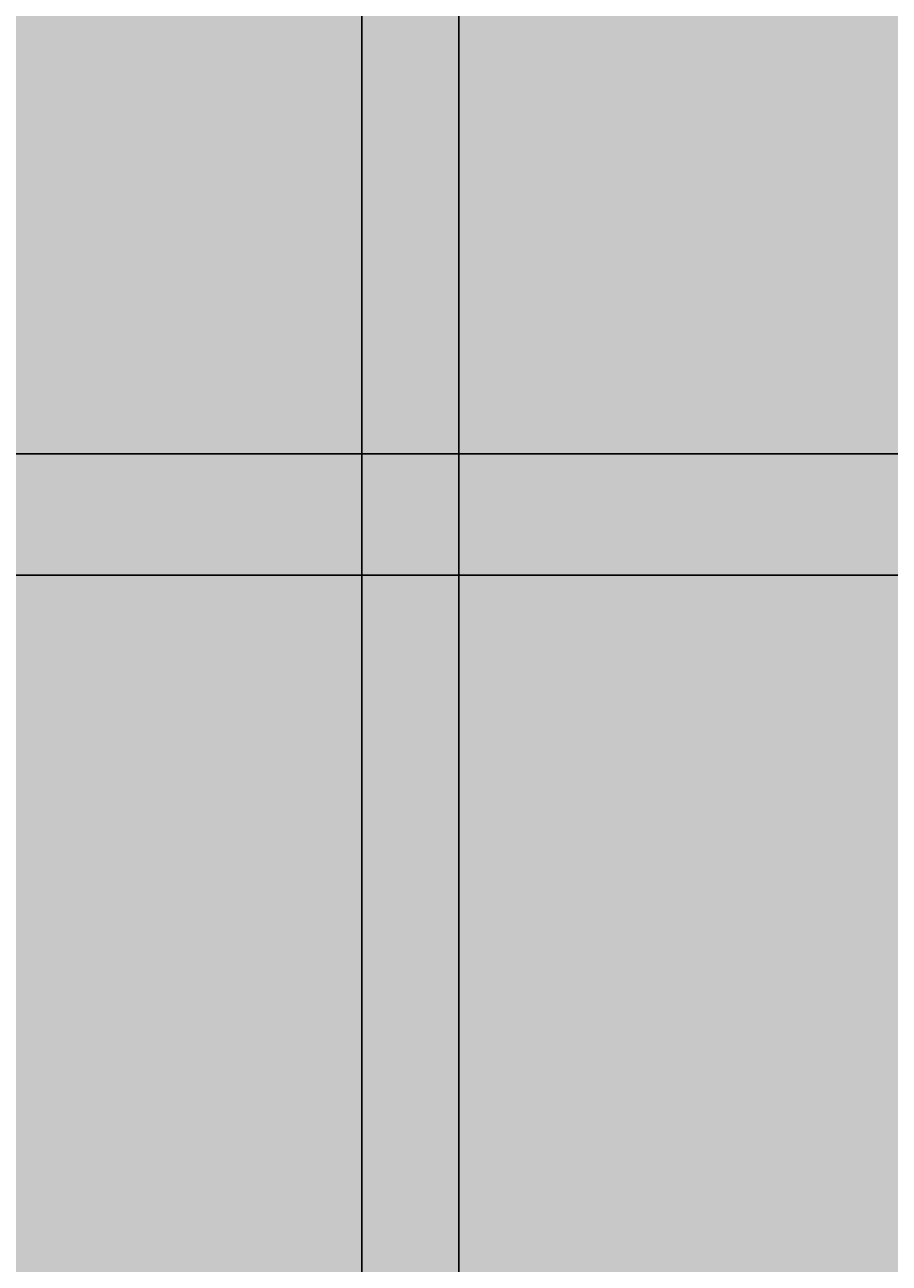
# Model space of a CAD drawing. Units: inches. Extents: x -12 to 334, y -10 to 186.
# Tile 65 of 77: x 239 to 257, y 111 to 137. Entities that reach past the tile are written whole.
import ezdxf

# ---------------------------------------------------------------- set-up
doc = ezdxf.new("R2010")
doc.units = ezdxf.units.IN
doc.header["$MEASUREMENT"] = 0
doc.layers.add('M-DIMS', color=2, linetype='Continuous', lineweight=18)
doc.layers.add('M-EQPM-PATT', color=8, linetype='Continuous', lineweight=18)
doc.styles.get("Standard").update_dxf_attribs({"font": 'arial.ttf'})
doc.dimstyles.get("Standard").update_dxf_attribs({"dimtxt": 0.18, "dimasz": 0.18, "dimexe": 0.18, "dimexo": 0.0625, "dimgap": 0.09, "dimtad": 0, "dimtih": 1, "dimtoh": 1, "dimdec": 4, "dimzin": 0, "dimdsep": 46, "dimtxsty": 'Standard', "dimcen": 0.09, "dimadec": 0, "dimazin": 0, "dimtfac": 1, "dimtdec": 4, "dimtofl": 0, "dimtmove": 0, "dimatfit": 3, "dimfxl": 1, "dimtolj": 1, "dimtzin": 0, "dimarcsym": 0})

# ---------------------------------------------------------------- blocks, each defined once
blk = doc.blocks.new('*D5')
at = {"layer": 'Defpoints', "color": 0, "transparency": 16777216}
for p in [(58.1, 127.708), (58.1, 125.208), (295.976, 125.208)]:
    blk.add_point(p, dxfattribs=at)
at = {"layer": 'M-DIMS', "color": 0, "lineweight": -2, "transparency": 16777216}
for p, q in [((58.163, 127.708), (296.156, 127.708)), ((295.976, 127.528), (295.976, 126.64)), ((295.976, 125.388), (295.976, 126.276)), ((58.163, 125.208), (296.156, 125.208))]:
    blk.add_line(p, q, dxfattribs=at)
at = {"layer": 'M-DIMS', "color": 0, "transparency": 16777216}
for points in [[(295.946, 127.528), (296.006, 127.528), (295.976, 127.708)], [(295.946, 125.388), (296.006, 125.388), (295.976, 125.208)]]:
    blk.add_solid(points, dxfattribs=at)
at = {"layer": 'M-DIMS', "color": 0, "transparency": 16777216, "insert": (295.976, 126.458), "char_height": 0.18, "attachment_point": 5}
blk.add_mtext('\\A1;2.5', dxfattribs=at)
blk = doc.blocks.new('*D36')
at = {"layer": 'Defpoints', "color": 0, "transparency": 16777216}
for p in [(247.935, 169.385), (245.935, 82.697), (247.935, 82.697)]:
    blk.add_point(p, dxfattribs=at)
at = {"layer": 'M-DIMS', "color": 0, "lineweight": -2, "transparency": 16777216}
for p, q in [((245.935, 82.759), (245.935, 169.565)), ((247.935, 82.759), (247.935, 169.565)), ((246.115, 169.385), (246.786, 169.385)), ((247.755, 169.385), (247.085, 169.385))]:
    blk.add_line(p, q, dxfattribs=at)
at = {"layer": 'M-DIMS', "color": 0, "transparency": 16777216}
for points in [[(246.115, 169.415), (246.115, 169.355), (245.935, 169.385)], [(247.755, 169.415), (247.755, 169.355), (247.935, 169.385)]]:
    blk.add_solid(points, dxfattribs=at)
at = {"layer": 'M-DIMS', "color": 0, "transparency": 16777216, "insert": (246.935, 169.385), "char_height": 0.18, "attachment_point": 5}
blk.add_mtext('\\A1;2', dxfattribs=at)
blk = doc.blocks.new('*D37')
at = {"layer": 'Defpoints', "color": 0, "transparency": 16777216}
for p in [(245.935, 169.385), (232.576, 46.854), (245.935, 46.854)]:
    blk.add_point(p, dxfattribs=at)
at = {"layer": 'M-DIMS', "color": 0, "lineweight": -2, "transparency": 16777216}
for p, q in [((232.576, 46.917), (232.576, 169.565)), ((245.935, 46.917), (245.935, 169.565)), ((232.756, 169.385), (238.871, 169.385)), ((245.755, 169.385), (239.641, 169.385))]:
    blk.add_line(p, q, dxfattribs=at)
at = {"layer": 'M-DIMS', "color": 0, "transparency": 16777216}
for points in [[(232.756, 169.415), (232.756, 169.355), (232.576, 169.385)], [(245.755, 169.415), (245.755, 169.355), (245.935, 169.385)]]:
    blk.add_solid(points, dxfattribs=at)
at = {"layer": 'M-DIMS', "color": 0, "transparency": 16777216, "insert": (239.256, 169.385), "char_height": 0.18, "attachment_point": 5}
blk.add_mtext('\\A1;13.36', dxfattribs=at)
blk = doc.blocks.new('*D40')
at = {"layer": 'Defpoints', "color": 0, "transparency": 16777216}
for p in [(278.229, 116.208), (187.394, 91.899)]:
    blk.add_point(p, dxfattribs=at)
at = {"layer": 'M-DIMS', "color": 0, "lineweight": -2, "transparency": 16777216}
for p, q in [((332.73, 130.793), (278.403, 116.254)), ((187.394, 91.809), (187.394, 91.989)), ((187.304, 91.899), (187.484, 91.899))]:
    blk.add_line(p, q, dxfattribs=at)
at = {"layer": 'M-DIMS', "color": 0, "transparency": 16777216}
blk.add_solid([(278.395, 116.283), (278.411, 116.225), (278.229, 116.208)], dxfattribs=at)
at = {"layer": 'M-DIMS', "color": 0, "transparency": 16777216, "insert": (333.21, 130.793), "char_height": 0.18, "attachment_point": 5}
blk.add_mtext('\\A1;R94.03', dxfattribs=at)

msp = doc.modelspace()

# ---------------------------------------------------------------- hatches: boundary and pattern name
at = {"layer": 'M-EQPM-PATT', "transparency": 33554556}
h = msp.add_hatch(color=256, dxfattribs=at)
h.set_gradient(color1=(248, 206, 179), color2=(248, 206, 179), tint=1)
h.paths.add_polyline_path([(179.7818, 136.8871), (126.9567, 136.8871), (106.1771, 100.8958), (171.5458, 100.8958)])
h.paths.add_polyline_path([(268.3808, 136.9435), (214.0166, 136.9435), (214.0166, 154.8345), (196.3421, 154.8345), (196.3421, 136.8871), (179.7818, 136.8871), (171.5458, 100.8958), (231.7758, 100.8958, -0.4142136), (251.9801, 80.6915), (279.7263, 80.6915, 0.1631825)])

# ---------------------------------------------------------------- dimensions: what is measured, and where the dimension line sits
at = {"layer": 'M-DIMS'}
for base, p1, p2, override, picture, middle in [((245.9354, 169.3845), (232.5761, 46.8541), (245.9354, 46.8541), {"dimdec": 2, "dimlfac": 1, "dimrnd": 0, "dimzin": 0, "dimdsep": 46, "dimlunit": 2}, '*D37', (239.2558, 169.3845)), ((247.9354, 169.3845), (245.9354, 82.6969), (247.9354, 82.6969), {"dimdec": 0, "dimlfac": 1, "dimrnd": 0, "dimzin": 0, "dimdsep": 46, "dimlunit": 2}, '*D36', (246.9354, 169.3845))]:
    dim = msp.add_linear_dim(base=base, p1=p1, p2=p2, dimstyle='Standard', override=override, dxfattribs=at)
    dim.commit()
    dim.dimension.update_dxf_attribs({"geometry": picture, "text_midpoint": middle})
dim = msp.add_radius_dim(center=(187.3936, 91.8988), mpoint=(278.2291, 116.2078), dimstyle='Standard', override={"dimdec": 2, "dimlfac": 1, "dimrnd": 0, "dimzin": 0, "dimdsep": 46, "dimlunit": 2}, dxfattribs=at)
dim.commit()
dim.dimension.update_dxf_attribs({"geometry": '*D40', "text_midpoint": (332.7304, 130.7932), "dimtype": 164})
dim = msp.add_linear_dim(base=(295.9756, 125.2078), p1=(58.1002, 127.7078), p2=(58.1002, 125.2078), angle=90, dimstyle='Standard', override={"dimdec": 1, "dimlfac": 1, "dimrnd": 0, "dimzin": 0, "dimdsep": 46, "dimlunit": 2}, dxfattribs=at)
dim.commit()
dim.dimension.update_dxf_attribs({"geometry": '*D5', "text_midpoint": (295.9756, 126.4578)})

doc.saveas('drawing.dxf')
